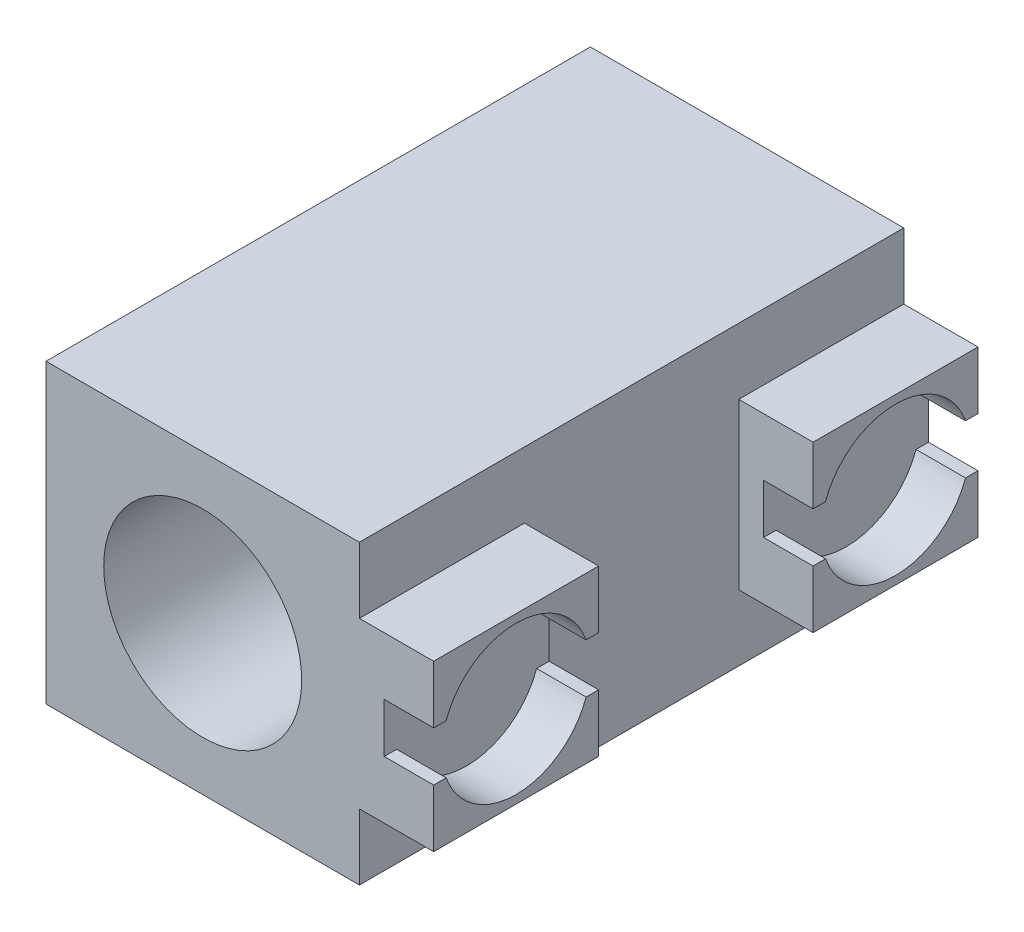
ISO-10303-21;
HEADER;
FILE_DESCRIPTION(('STEP AP214'),'2;1');
FILE_NAME('part.step','',(''),(''),'','','');
FILE_SCHEMA(('AUTOMOTIVE_DESIGN { 1 0 10303 214 1 1 1 1 }'));
ENDSEC;
DATA;
#1=APPLICATION_CONTEXT('core data for automotive mechanical design processes');
#2=APPLICATION_PROTOCOL_DEFINITION('international standard','automotive_design',2000,#1);
#3=PRODUCT_CONTEXT('',#1,'mechanical');
#4=PRODUCT('Part','Part','',(#3));
#5=PRODUCT_RELATED_PRODUCT_CATEGORY('part','',(#4));
#6=PRODUCT_DEFINITION_FORMATION('','',#4);
#7=PRODUCT_DEFINITION_CONTEXT('part definition',#1,'design');
#8=PRODUCT_DEFINITION('design','',#6,#7);
#9=PRODUCT_DEFINITION_SHAPE('','',#8);
#10=(LENGTH_UNIT() NAMED_UNIT(*) SI_UNIT(.MILLI.,.METRE.));
#11=(NAMED_UNIT(*) PLANE_ANGLE_UNIT() SI_UNIT($,.RADIAN.));
#12=(NAMED_UNIT(*) SI_UNIT($,.STERADIAN.) SOLID_ANGLE_UNIT());
#13=UNCERTAINTY_MEASURE_WITH_UNIT(LENGTH_MEASURE(1.E-05),#10,'distance_accuracy_value','');
#14=(GEOMETRIC_REPRESENTATION_CONTEXT(3) GLOBAL_UNCERTAINTY_ASSIGNED_CONTEXT((#13)) GLOBAL_UNIT_ASSIGNED_CONTEXT((#10,
#11,#12)) REPRESENTATION_CONTEXT('',''));
#15=CARTESIAN_POINT('',(0.,0.,0.));
#16=DIRECTION('',(0.,0.,1.));
#17=DIRECTION('',(1.,0.,0.));
#18=AXIS2_PLACEMENT_3D('',#15,#16,#17);
#19=CARTESIAN_POINT('',(47.,0.,0.));
#20=DIRECTION('',(1.,0.,0.));
#21=DIRECTION('',(0.,0.,-1.));
#22=AXIS2_PLACEMENT_3D('',#19,#20,#21);
#23=PLANE('',#22);
#24=DIRECTION('',(0.,0.,1.));
#25=VECTOR('',#24,1.);
#26=CARTESIAN_POINT('',(47.,-3.,-19.));
#27=LINE('',#26,#25);
#28=CARTESIAN_POINT('',(47.,-3.,-14.5147186257614));
#29=VERTEX_POINT('',#28);
#30=CARTESIAN_POINT('',(47.,-3.,-13.));
#31=VERTEX_POINT('',#30);
#32=EDGE_CURVE('E445',#29,#31,#27,.T.);
#33=ORIENTED_EDGE('',*,*,#32,.T.);
#34=DIRECTION('',(0.,-1.,0.));
#35=VECTOR('',#34,1.);
#36=CARTESIAN_POINT('',(47.,10.,-13.));
#37=LINE('',#36,#35);
#38=CARTESIAN_POINT('',(47.,-9.99999999999999,-13.));
#39=VERTEX_POINT('',#38);
#40=EDGE_CURVE('E258',#31,#39,#37,.T.);
#41=ORIENTED_EDGE('',*,*,#40,.T.);
#42=DIRECTION('',(0.,0.,-1.));
#43=VECTOR('',#42,1.);
#44=CARTESIAN_POINT('',(47.,-9.99999999999999,-13.));
#45=LINE('',#44,#43);
#46=CARTESIAN_POINT('',(47.,-9.99999999999999,-33.));
#47=VERTEX_POINT('',#46);
#48=EDGE_CURVE('E275',#39,#47,#45,.T.);
#49=ORIENTED_EDGE('',*,*,#48,.T.);
#50=DIRECTION('',(0.,1.,0.));
#51=VECTOR('',#50,1.);
#52=CARTESIAN_POINT('',(47.,-9.99999999999999,-33.));
#53=LINE('',#52,#51);
#54=CARTESIAN_POINT('',(47.,-3.,-33.));
#55=VERTEX_POINT('',#54);
#56=EDGE_CURVE('E421',#47,#55,#53,.T.);
#57=ORIENTED_EDGE('',*,*,#56,.T.);
#58=DIRECTION('',(0.,0.,-1.));
#59=VECTOR('',#58,1.);
#60=CARTESIAN_POINT('',(47.,-3.,-27.));
#61=LINE('',#60,#59);
#62=CARTESIAN_POINT('',(47.,-3.,-31.4852813742386));
#63=VERTEX_POINT('',#62);
#64=EDGE_CURVE('E463',#63,#55,#61,.T.);
#65=ORIENTED_EDGE('',*,*,#64,.F.);
#66=CARTESIAN_POINT('',(47.,0.,-23.));
#67=DIRECTION('',(1.,0.,0.));
#68=DIRECTION('',(0.,0.,-1.));
#69=AXIS2_PLACEMENT_3D('',#66,#67,#68);
#70=CIRCLE('',#69,9.);
#71=EDGE_CURVE('E475',#29,#63,#70,.T.);
#72=ORIENTED_EDGE('',*,*,#71,.F.);
#73=EDGE_LOOP('',(#33,#41,#49,#57,#65,#72));
#74=FACE_BOUND('',#73,.T.);
#75=ADVANCED_FACE('F39',(#74),#23,.T.);
#76=CARTESIAN_POINT('',(41.,0.,-23.));
#77=DIRECTION('',(1.,0.,0.));
#78=DIRECTION('',(0.,0.,-1.));
#79=AXIS2_PLACEMENT_3D('',#76,#77,#78);
#80=CYLINDRICAL_SURFACE('',#79,9.);
#81=CARTESIAN_POINT('',(41.,0.,-23.));
#82=DIRECTION('',(1.,0.,0.));
#83=DIRECTION('',(0.,0.,-1.));
#84=AXIS2_PLACEMENT_3D('',#81,#82,#83);
#85=CIRCLE('',#84,9.);
#86=CARTESIAN_POINT('',(41.,-3.,-14.5147186257614));
#87=VERTEX_POINT('',#86);
#88=CARTESIAN_POINT('',(41.,-3.,-31.4852813742386));
#89=VERTEX_POINT('',#88);
#90=EDGE_CURVE('E476',#87,#89,#85,.T.);
#91=ORIENTED_EDGE('',*,*,#90,.F.);
#92=DIRECTION('',(1.,0.,0.));
#93=VECTOR('',#92,1.);
#94=CARTESIAN_POINT('',(41.,-3.,-14.5147186257614));
#95=LINE('',#94,#93);
#96=EDGE_CURVE('E454',#87,#29,#95,.T.);
#97=ORIENTED_EDGE('',*,*,#96,.T.);
#98=ORIENTED_EDGE('',*,*,#71,.T.);
#99=DIRECTION('',(1.,0.,0.));
#100=VECTOR('',#99,1.);
#101=CARTESIAN_POINT('',(41.,-3.,-31.4852813742386));
#102=LINE('',#101,#100);
#103=EDGE_CURVE('E473',#63,#89,#102,.F.);
#104=ORIENTED_EDGE('',*,*,#103,.T.);
#105=EDGE_LOOP('',(#91,#97,#98,#104));
#106=FACE_BOUND('',#105,.T.);
#107=ADVANCED_FACE('F543',(#106),#80,.F.);
#108=CARTESIAN_POINT('',(47.,0.,0.));
#109=DIRECTION('',(-1.,0.,0.));
#110=DIRECTION('',(0.,0.,1.));
#111=AXIS2_PLACEMENT_3D('',#108,#109,#110);
#112=PLANE('',#111);
#113=DIRECTION('',(0.,1.,0.));
#114=VECTOR('',#113,1.);
#115=CARTESIAN_POINT('',(47.,10.,13.));
#116=LINE('',#115,#114);
#117=CARTESIAN_POINT('',(47.,-9.99999999999999,13.));
#118=VERTEX_POINT('',#117);
#119=CARTESIAN_POINT('',(47.,-3.,13.));
#120=VERTEX_POINT('',#119);
#121=EDGE_CURVE('E289',#118,#120,#116,.T.);
#122=ORIENTED_EDGE('',*,*,#121,.T.);
#123=DIRECTION('',(0.,0.,-1.));
#124=VECTOR('',#123,1.);
#125=CARTESIAN_POINT('',(47.,-3.,19.));
#126=LINE('',#125,#124);
#127=CARTESIAN_POINT('',(47.,-3.,14.5147186257614));
#128=VERTEX_POINT('',#127);
#129=EDGE_CURVE('E491',#128,#120,#126,.T.);
#130=ORIENTED_EDGE('',*,*,#129,.F.);
#131=CARTESIAN_POINT('',(47.,0.,23.));
#132=DIRECTION('',(1.,0.,0.));
#133=DIRECTION('',(0.,0.,-1.));
#134=AXIS2_PLACEMENT_3D('',#131,#132,#133);
#135=CIRCLE('',#134,9.);
#136=CARTESIAN_POINT('',(47.,-3.,31.4852813742386));
#137=VERTEX_POINT('',#136);
#138=EDGE_CURVE('E416',#137,#128,#135,.T.);
#139=ORIENTED_EDGE('',*,*,#138,.F.);
#140=DIRECTION('',(0.,0.,-1.));
#141=VECTOR('',#140,1.);
#142=CARTESIAN_POINT('',(47.,-3.,226.327850741589));
#143=LINE('',#142,#141);
#144=CARTESIAN_POINT('',(47.,-3.,33.));
#145=VERTEX_POINT('',#144);
#146=EDGE_CURVE('E376',#145,#137,#143,.T.);
#147=ORIENTED_EDGE('',*,*,#146,.F.);
#148=DIRECTION('',(0.,-1.,0.));
#149=VECTOR('',#148,1.);
#150=CARTESIAN_POINT('',(47.,-10.,33.));
#151=LINE('',#150,#149);
#152=CARTESIAN_POINT('',(47.,-10.,33.));
#153=VERTEX_POINT('',#152);
#154=EDGE_CURVE('E281',#145,#153,#151,.T.);
#155=ORIENTED_EDGE('',*,*,#154,.T.);
#156=DIRECTION('',(0.,0.,-1.));
#157=VECTOR('',#156,1.);
#158=CARTESIAN_POINT('',(47.,-9.99999999999999,13.));
#159=LINE('',#158,#157);
#160=EDGE_CURVE('E285',#153,#118,#159,.T.);
#161=ORIENTED_EDGE('',*,*,#160,.T.);
#162=EDGE_LOOP('',(#122,#130,#139,#147,#155,#161));
#163=FACE_BOUND('',#162,.T.);
#164=ADVANCED_FACE('F375',(#163),#112,.F.);
#165=CARTESIAN_POINT('',(41.,0.,23.));
#166=DIRECTION('',(1.,0.,0.));
#167=DIRECTION('',(0.,0.,-1.));
#168=AXIS2_PLACEMENT_3D('',#165,#166,#167);
#169=CYLINDRICAL_SURFACE('',#168,9.);
#170=ORIENTED_EDGE('',*,*,#138,.T.);
#171=DIRECTION('',(1.,0.,0.));
#172=VECTOR('',#171,1.);
#173=CARTESIAN_POINT('',(41.,-3.,14.5147186257614));
#174=LINE('',#173,#172);
#175=CARTESIAN_POINT('',(41.,-3.,14.5147186257614));
#176=VERTEX_POINT('',#175);
#177=EDGE_CURVE('E390',#128,#176,#174,.F.);
#178=ORIENTED_EDGE('',*,*,#177,.T.);
#179=CARTESIAN_POINT('',(41.,0.,23.));
#180=DIRECTION('',(1.,0.,0.));
#181=DIRECTION('',(0.,0.,-1.));
#182=AXIS2_PLACEMENT_3D('',#179,#180,#181);
#183=CIRCLE('',#182,9.);
#184=CARTESIAN_POINT('',(41.,-3.,31.4852813742386));
#185=VERTEX_POINT('',#184);
#186=EDGE_CURVE('E268',#185,#176,#183,.T.);
#187=ORIENTED_EDGE('',*,*,#186,.F.);
#188=DIRECTION('',(1.,0.,0.));
#189=VECTOR('',#188,1.);
#190=CARTESIAN_POINT('',(41.,-3.,31.4852813742386));
#191=LINE('',#190,#189);
#192=EDGE_CURVE('E414',#137,#185,#191,.F.);
#193=ORIENTED_EDGE('',*,*,#192,.F.);
#194=EDGE_LOOP('',(#170,#178,#187,#193));
#195=FACE_BOUND('',#194,.T.);
#196=ADVANCED_FACE('F530',(#195),#169,.F.);
#197=CARTESIAN_POINT('',(47.,3.,14.5147186257614));
#198=VERTEX_POINT('',#197);
#199=CARTESIAN_POINT('',(47.,3.,31.4852813742386));
#200=VERTEX_POINT('',#199);
#201=EDGE_CURVE('E415',#198,#200,#135,.T.);
#202=ORIENTED_EDGE('',*,*,#201,.F.);
#203=DIRECTION('',(0.,0.,-1.));
#204=VECTOR('',#203,1.);
#205=CARTESIAN_POINT('',(47.,3.,19.));
#206=LINE('',#205,#204);
#207=CARTESIAN_POINT('',(47.,3.,13.));
#208=VERTEX_POINT('',#207);
#209=EDGE_CURVE('E492',#198,#208,#206,.T.);
#210=ORIENTED_EDGE('',*,*,#209,.T.);
#211=CARTESIAN_POINT('',(47.,10.,13.));
#212=VERTEX_POINT('',#211);
#213=EDGE_CURVE('E288',#208,#212,#116,.T.);
#214=ORIENTED_EDGE('',*,*,#213,.T.);
#215=DIRECTION('',(0.,0.,1.));
#216=VECTOR('',#215,1.);
#217=CARTESIAN_POINT('',(47.,10.,33.));
#218=LINE('',#217,#216);
#219=CARTESIAN_POINT('',(47.,10.,33.));
#220=VERTEX_POINT('',#219);
#221=EDGE_CURVE('E286',#212,#220,#218,.T.);
#222=ORIENTED_EDGE('',*,*,#221,.T.);
#223=CARTESIAN_POINT('',(47.,3.,33.));
#224=VERTEX_POINT('',#223);
#225=EDGE_CURVE('E278',#220,#224,#151,.T.);
#226=ORIENTED_EDGE('',*,*,#225,.T.);
#227=DIRECTION('',(0.,0.,-1.));
#228=VECTOR('',#227,1.);
#229=CARTESIAN_POINT('',(47.,3.,226.327850741589));
#230=LINE('',#229,#228);
#231=EDGE_CURVE('E400',#224,#200,#230,.T.);
#232=ORIENTED_EDGE('',*,*,#231,.T.);
#233=EDGE_LOOP('',(#202,#210,#214,#222,#226,#232));
#234=FACE_BOUND('',#233,.T.);
#235=ADVANCED_FACE('F503',(#234),#112,.F.);
#236=CARTESIAN_POINT('',(41.,3.,14.5147186257614));
#237=VERTEX_POINT('',#236);
#238=CARTESIAN_POINT('',(41.,3.,31.4852813742386));
#239=VERTEX_POINT('',#238);
#240=EDGE_CURVE('E417',#237,#239,#183,.T.);
#241=ORIENTED_EDGE('',*,*,#240,.F.);
#242=DIRECTION('',(1.,0.,0.));
#243=VECTOR('',#242,1.);
#244=CARTESIAN_POINT('',(41.,3.,14.5147186257614));
#245=LINE('',#244,#243);
#246=EDGE_CURVE('E394',#237,#198,#245,.T.);
#247=ORIENTED_EDGE('',*,*,#246,.T.);
#248=ORIENTED_EDGE('',*,*,#201,.T.);
#249=DIRECTION('',(1.,0.,0.));
#250=VECTOR('',#249,1.);
#251=CARTESIAN_POINT('',(41.,3.,31.4852813742386));
#252=LINE('',#251,#250);
#253=EDGE_CURVE('E406',#239,#200,#252,.T.);
#254=ORIENTED_EDGE('',*,*,#253,.F.);
#255=EDGE_LOOP('',(#241,#247,#248,#254));
#256=FACE_BOUND('',#255,.T.);
#257=ADVANCED_FACE('F498',(#256),#169,.F.);
#258=CARTESIAN_POINT('',(38.,0.,0.));
#259=DIRECTION('',(1.,0.,0.));
#260=DIRECTION('',(0.,0.,-1.));
#261=AXIS2_PLACEMENT_3D('',#258,#259,#260);
#262=PLANE('',#261);
#263=DIRECTION('',(0.,1.,0.));
#264=VECTOR('',#263,1.);
#265=CARTESIAN_POINT('',(38.,18.,-33.));
#266=LINE('',#265,#264);
#267=CARTESIAN_POINT('',(38.,-18.,-33.));
#268=VERTEX_POINT('',#267);
#269=CARTESIAN_POINT('',(38.,-9.99999999999999,-33.));
#270=VERTEX_POINT('',#269);
#271=EDGE_CURVE('E311',#268,#270,#266,.T.);
#272=ORIENTED_EDGE('',*,*,#271,.T.);
#273=DIRECTION('',(0.,0.,-1.));
#274=VECTOR('',#273,1.);
#275=CARTESIAN_POINT('',(38.,-9.99999999999999,-13.));
#276=LINE('',#275,#274);
#277=CARTESIAN_POINT('',(38.,-9.99999999999999,-13.));
#278=VERTEX_POINT('',#277);
#279=EDGE_CURVE('E262',#278,#270,#276,.T.);
#280=ORIENTED_EDGE('',*,*,#279,.F.);
#281=DIRECTION('',(0.,-1.,0.));
#282=VECTOR('',#281,1.);
#283=CARTESIAN_POINT('',(38.,10.,-13.));
#284=LINE('',#283,#282);
#285=CARTESIAN_POINT('',(38.,10.,-13.));
#286=VERTEX_POINT('',#285);
#287=EDGE_CURVE('E271',#286,#278,#284,.T.);
#288=ORIENTED_EDGE('',*,*,#287,.F.);
#289=DIRECTION('',(0.,0.,1.));
#290=VECTOR('',#289,1.);
#291=CARTESIAN_POINT('',(38.,10.,-33.));
#292=LINE('',#291,#290);
#293=CARTESIAN_POINT('',(38.,10.,-33.));
#294=VERTEX_POINT('',#293);
#295=EDGE_CURVE('E270',#294,#286,#292,.T.);
#296=ORIENTED_EDGE('',*,*,#295,.F.);
#297=CARTESIAN_POINT('',(38.,18.,-33.));
#298=VERTEX_POINT('',#297);
#299=EDGE_CURVE('E320',#294,#298,#266,.T.);
#300=ORIENTED_EDGE('',*,*,#299,.T.);
#301=DIRECTION('',(0.,0.,1.));
#302=VECTOR('',#301,1.);
#303=CARTESIAN_POINT('',(38.,18.,33.));
#304=LINE('',#303,#302);
#305=CARTESIAN_POINT('',(38.,18.,33.));
#306=VERTEX_POINT('',#305);
#307=EDGE_CURVE('E316',#298,#306,#304,.T.);
#308=ORIENTED_EDGE('',*,*,#307,.T.);
#309=DIRECTION('',(0.,-1.,0.));
#310=VECTOR('',#309,1.);
#311=CARTESIAN_POINT('',(38.,18.,33.));
#312=LINE('',#311,#310);
#313=CARTESIAN_POINT('',(38.,10.,33.));
#314=VERTEX_POINT('',#313);
#315=EDGE_CURVE('E319',#306,#314,#312,.T.);
#316=ORIENTED_EDGE('',*,*,#315,.T.);
#317=DIRECTION('',(0.,0.,1.));
#318=VECTOR('',#317,1.);
#319=CARTESIAN_POINT('',(38.,10.,33.));
#320=LINE('',#319,#318);
#321=CARTESIAN_POINT('',(38.,10.,13.));
#322=VERTEX_POINT('',#321);
#323=EDGE_CURVE('E300',#322,#314,#320,.T.);
#324=ORIENTED_EDGE('',*,*,#323,.F.);
#325=DIRECTION('',(0.,1.,0.));
#326=VECTOR('',#325,1.);
#327=CARTESIAN_POINT('',(38.,10.,13.));
#328=LINE('',#327,#326);
#329=CARTESIAN_POINT('',(38.,-9.99999999999999,13.));
#330=VERTEX_POINT('',#329);
#331=EDGE_CURVE('E293',#330,#322,#328,.T.);
#332=ORIENTED_EDGE('',*,*,#331,.F.);
#333=DIRECTION('',(0.,0.,-1.));
#334=VECTOR('',#333,1.);
#335=CARTESIAN_POINT('',(38.,-9.99999999999999,13.));
#336=LINE('',#335,#334);
#337=CARTESIAN_POINT('',(38.,-10.,33.));
#338=VERTEX_POINT('',#337);
#339=EDGE_CURVE('E276',#338,#330,#336,.T.);
#340=ORIENTED_EDGE('',*,*,#339,.F.);
#341=CARTESIAN_POINT('',(38.,-18.,33.));
#342=VERTEX_POINT('',#341);
#343=EDGE_CURVE('E317',#338,#342,#312,.T.);
#344=ORIENTED_EDGE('',*,*,#343,.T.);
#345=DIRECTION('',(0.,0.,-1.));
#346=VECTOR('',#345,1.);
#347=CARTESIAN_POINT('',(38.,-18.,33.));
#348=LINE('',#347,#346);
#349=EDGE_CURVE('E325',#342,#268,#348,.T.);
#350=ORIENTED_EDGE('',*,*,#349,.T.);
#351=EDGE_LOOP('',(#272,#280,#288,#296,#300,#308,#316,#324,#332,#340,#344,#350));
#352=FACE_BOUND('',#351,.T.);
#353=ADVANCED_FACE('F362',(#352),#262,.T.);
#354=CARTESIAN_POINT('',(38.,18.,-33.));
#355=DIRECTION('',(0.,0.,1.));
#356=DIRECTION('',(1.,0.,0.));
#357=AXIS2_PLACEMENT_3D('',#354,#355,#356);
#358=PLANE('',#357);
#359=CARTESIAN_POINT('',(19.,0.,-33.));
#360=DIRECTION('',(0.,0.,1.));
#361=DIRECTION('',(1.,0.,0.));
#362=AXIS2_PLACEMENT_3D('',#359,#360,#361);
#363=CIRCLE('',#362,12.);
#364=CARTESIAN_POINT('',(31.,0.,-33.));
#365=VERTEX_POINT('',#364);
#366=EDGE_CURVE('E250',#365,#365,#363,.T.);
#367=ORIENTED_EDGE('',*,*,#366,.T.);
#368=EDGE_LOOP('',(#367));
#369=FACE_BOUND('',#368,.T.);
#370=DIRECTION('',(0.,1.,0.));
#371=VECTOR('',#370,1.);
#372=CARTESIAN_POINT('',(41.,0.,-33.));
#373=LINE('',#372,#371);
#374=CARTESIAN_POINT('',(41.,-3.,-33.));
#375=VERTEX_POINT('',#374);
#376=CARTESIAN_POINT('',(41.,3.,-33.));
#377=VERTEX_POINT('',#376);
#378=EDGE_CURVE('E451',#375,#377,#373,.T.);
#379=ORIENTED_EDGE('',*,*,#378,.F.);
#380=DIRECTION('',(-1.,0.,0.));
#381=VECTOR('',#380,1.);
#382=CARTESIAN_POINT('',(47.,-3.,-33.));
#383=LINE('',#382,#381);
#384=EDGE_CURVE('E459',#55,#375,#383,.T.);
#385=ORIENTED_EDGE('',*,*,#384,.F.);
#386=ORIENTED_EDGE('',*,*,#56,.F.);
#387=DIRECTION('',(-1.,0.,0.));
#388=VECTOR('',#387,1.);
#389=CARTESIAN_POINT('',(47.,-9.99999999999999,-33.));
#390=LINE('',#389,#388);
#391=EDGE_CURVE('E280',#47,#270,#390,.T.);
#392=ORIENTED_EDGE('',*,*,#391,.T.);
#393=ORIENTED_EDGE('',*,*,#271,.F.);
#394=DIRECTION('',(-1.,0.,0.));
#395=VECTOR('',#394,1.);
#396=CARTESIAN_POINT('',(38.,-18.,-33.));
#397=LINE('',#396,#395);
#398=CARTESIAN_POINT('',(0.,-18.,-33.));
#399=VERTEX_POINT('',#398);
#400=EDGE_CURVE('E322',#268,#399,#397,.T.);
#401=ORIENTED_EDGE('',*,*,#400,.T.);
#402=DIRECTION('',(0.,1.,0.));
#403=VECTOR('',#402,1.);
#404=CARTESIAN_POINT('',(0.,18.,-33.));
#405=LINE('',#404,#403);
#406=CARTESIAN_POINT('',(0.,18.,-33.));
#407=VERTEX_POINT('',#406);
#408=EDGE_CURVE('E315',#399,#407,#405,.T.);
#409=ORIENTED_EDGE('',*,*,#408,.T.);
#410=DIRECTION('',(-1.,0.,0.));
#411=VECTOR('',#410,1.);
#412=CARTESIAN_POINT('',(38.,18.,-33.));
#413=LINE('',#412,#411);
#414=EDGE_CURVE('E11',#298,#407,#413,.T.);
#415=ORIENTED_EDGE('',*,*,#414,.F.);
#416=ORIENTED_EDGE('',*,*,#299,.F.);
#417=DIRECTION('',(-1.,0.,0.));
#418=VECTOR('',#417,1.);
#419=CARTESIAN_POINT('',(47.,10.,-33.));
#420=LINE('',#419,#418);
#421=CARTESIAN_POINT('',(47.,10.,-33.));
#422=VERTEX_POINT('',#421);
#423=EDGE_CURVE('E274',#422,#294,#420,.T.);
#424=ORIENTED_EDGE('',*,*,#423,.F.);
#425=CARTESIAN_POINT('',(47.,3.,-33.));
#426=VERTEX_POINT('',#425);
#427=EDGE_CURVE('E425',#426,#422,#53,.T.);
#428=ORIENTED_EDGE('',*,*,#427,.F.);
#429=DIRECTION('',(1.,0.,0.));
#430=VECTOR('',#429,1.);
#431=CARTESIAN_POINT('',(41.,3.,-33.));
#432=LINE('',#431,#430);
#433=EDGE_CURVE('E460',#377,#426,#432,.T.);
#434=ORIENTED_EDGE('',*,*,#433,.F.);
#435=EDGE_LOOP('',(#379,#385,#386,#392,#393,#401,#409,#415,#416,#424,#428,#434));
#436=FACE_BOUND('',#435,.T.);
#437=ADVANCED_FACE('F41',(#369,#436),#358,.F.);
#438=CARTESIAN_POINT('',(38.,18.,33.));
#439=DIRECTION('',(0.,-1.,0.));
#440=DIRECTION('',(0.,0.,-1.));
#441=AXIS2_PLACEMENT_3D('',#438,#439,#440);
#442=PLANE('',#441);
#443=DIRECTION('',(0.,0.,1.));
#444=VECTOR('',#443,1.);
#445=CARTESIAN_POINT('',(0.,18.,33.));
#446=LINE('',#445,#444);
#447=CARTESIAN_POINT('',(0.,18.,33.));
#448=VERTEX_POINT('',#447);
#449=EDGE_CURVE('E330',#407,#448,#446,.T.);
#450=ORIENTED_EDGE('',*,*,#449,.T.);
#451=DIRECTION('',(-1.,0.,0.));
#452=VECTOR('',#451,1.);
#453=CARTESIAN_POINT('',(38.,18.,33.));
#454=LINE('',#453,#452);
#455=EDGE_CURVE('E50',#306,#448,#454,.T.);
#456=ORIENTED_EDGE('',*,*,#455,.F.);
#457=ORIENTED_EDGE('',*,*,#307,.F.);
#458=ORIENTED_EDGE('',*,*,#414,.T.);
#459=EDGE_LOOP('',(#450,#456,#457,#458));
#460=FACE_BOUND('',#459,.T.);
#461=ADVANCED_FACE('F535',(#460),#442,.F.);
#462=CARTESIAN_POINT('',(38.,18.,33.));
#463=DIRECTION('',(0.,0.,-1.));
#464=DIRECTION('',(-1.,0.,0.));
#465=AXIS2_PLACEMENT_3D('',#462,#463,#464);
#466=PLANE('',#465);
#467=CARTESIAN_POINT('',(19.,0.,33.));
#468=DIRECTION('',(0.,0.,1.));
#469=DIRECTION('',(1.,0.,0.));
#470=AXIS2_PLACEMENT_3D('',#467,#468,#469);
#471=CIRCLE('',#470,12.);
#472=CARTESIAN_POINT('',(31.,0.,33.));
#473=VERTEX_POINT('',#472);
#474=EDGE_CURVE('E797',#473,#473,#471,.T.);
#475=ORIENTED_EDGE('',*,*,#474,.F.);
#476=EDGE_LOOP('',(#475));
#477=FACE_BOUND('',#476,.T.);
#478=ORIENTED_EDGE('',*,*,#154,.F.);
#479=DIRECTION('',(-1.,0.,0.));
#480=VECTOR('',#479,1.);
#481=CARTESIAN_POINT('',(41.,-3.,33.));
#482=LINE('',#481,#480);
#483=CARTESIAN_POINT('',(41.,-3.,33.));
#484=VERTEX_POINT('',#483);
#485=EDGE_CURVE('E378',#145,#484,#482,.T.);
#486=ORIENTED_EDGE('',*,*,#485,.T.);
#487=DIRECTION('',(0.,1.,0.));
#488=VECTOR('',#487,1.);
#489=CARTESIAN_POINT('',(41.,0.,33.));
#490=LINE('',#489,#488);
#491=CARTESIAN_POINT('',(41.,0.,33.));
#492=VERTEX_POINT('',#491);
#493=EDGE_CURVE('E387',#484,#492,#490,.T.);
#494=ORIENTED_EDGE('',*,*,#493,.T.);
#495=DIRECTION('',(0.,1.,0.));
#496=VECTOR('',#495,1.);
#497=CARTESIAN_POINT('',(41.,0.,33.));
#498=LINE('',#497,#496);
#499=CARTESIAN_POINT('',(41.,3.,33.));
#500=VERTEX_POINT('',#499);
#501=EDGE_CURVE('E386',#492,#500,#498,.T.);
#502=ORIENTED_EDGE('',*,*,#501,.T.);
#503=DIRECTION('',(1.,0.,0.));
#504=VECTOR('',#503,1.);
#505=CARTESIAN_POINT('',(41.,3.,33.));
#506=LINE('',#505,#504);
#507=EDGE_CURVE('E399',#500,#224,#506,.T.);
#508=ORIENTED_EDGE('',*,*,#507,.T.);
#509=ORIENTED_EDGE('',*,*,#225,.F.);
#510=DIRECTION('',(-1.,0.,0.));
#511=VECTOR('',#510,1.);
#512=CARTESIAN_POINT('',(47.,10.,33.));
#513=LINE('',#512,#511);
#514=EDGE_CURVE('E295',#220,#314,#513,.T.);
#515=ORIENTED_EDGE('',*,*,#514,.T.);
#516=ORIENTED_EDGE('',*,*,#315,.F.);
#517=ORIENTED_EDGE('',*,*,#455,.T.);
#518=DIRECTION('',(0.,-1.,0.));
#519=VECTOR('',#518,1.);
#520=CARTESIAN_POINT('',(0.,18.,33.));
#521=LINE('',#520,#519);
#522=CARTESIAN_POINT('',(0.,-18.,33.));
#523=VERTEX_POINT('',#522);
#524=EDGE_CURVE('E328',#448,#523,#521,.T.);
#525=ORIENTED_EDGE('',*,*,#524,.T.);
#526=DIRECTION('',(-1.,0.,0.));
#527=VECTOR('',#526,1.);
#528=CARTESIAN_POINT('',(38.,-18.,33.));
#529=LINE('',#528,#527);
#530=EDGE_CURVE('E333',#342,#523,#529,.T.);
#531=ORIENTED_EDGE('',*,*,#530,.F.);
#532=ORIENTED_EDGE('',*,*,#343,.F.);
#533=DIRECTION('',(-1.,0.,0.));
#534=VECTOR('',#533,1.);
#535=CARTESIAN_POINT('',(47.,-10.,33.));
#536=LINE('',#535,#534);
#537=EDGE_CURVE('E310',#153,#338,#536,.T.);
#538=ORIENTED_EDGE('',*,*,#537,.F.);
#539=EDGE_LOOP('',(#478,#486,#494,#502,#508,#509,#515,#516,#517,#525,#531,#532,#538));
#540=FACE_BOUND('',#539,.T.);
#541=ADVANCED_FACE('F342',(#477,#540),#466,.F.);
#542=CARTESIAN_POINT('',(38.,-18.,33.));
#543=DIRECTION('',(0.,1.,0.));
#544=DIRECTION('',(0.,0.,1.));
#545=AXIS2_PLACEMENT_3D('',#542,#543,#544);
#546=PLANE('',#545);
#547=DIRECTION('',(0.,0.,-1.));
#548=VECTOR('',#547,1.);
#549=CARTESIAN_POINT('',(0.,-18.,33.));
#550=LINE('',#549,#548);
#551=EDGE_CURVE('E332',#523,#399,#550,.T.);
#552=ORIENTED_EDGE('',*,*,#551,.T.);
#553=ORIENTED_EDGE('',*,*,#400,.F.);
#554=ORIENTED_EDGE('',*,*,#349,.F.);
#555=ORIENTED_EDGE('',*,*,#530,.T.);
#556=EDGE_LOOP('',(#552,#553,#554,#555));
#557=FACE_BOUND('',#556,.T.);
#558=ADVANCED_FACE('F355',(#557),#546,.F.);
#559=CARTESIAN_POINT('',(0.,0.,0.));
#560=DIRECTION('',(1.,0.,0.));
#561=DIRECTION('',(0.,0.,-1.));
#562=AXIS2_PLACEMENT_3D('',#559,#560,#561);
#563=PLANE('',#562);
#564=ORIENTED_EDGE('',*,*,#408,.F.);
#565=ORIENTED_EDGE('',*,*,#551,.F.);
#566=ORIENTED_EDGE('',*,*,#524,.F.);
#567=ORIENTED_EDGE('',*,*,#449,.F.);
#568=EDGE_LOOP('',(#564,#565,#566,#567));
#569=FACE_BOUND('',#568,.T.);
#570=ADVANCED_FACE('F348',(#569),#563,.F.);
#571=CARTESIAN_POINT('',(47.,-9.99999999999999,13.));
#572=DIRECTION('',(0.,1.,0.));
#573=DIRECTION('',(0.,0.,1.));
#574=AXIS2_PLACEMENT_3D('',#571,#572,#573);
#575=PLANE('',#574);
#576=ORIENTED_EDGE('',*,*,#339,.T.);
#577=DIRECTION('',(-1.,0.,0.));
#578=VECTOR('',#577,1.);
#579=CARTESIAN_POINT('',(47.,-9.99999999999999,13.));
#580=LINE('',#579,#578);
#581=EDGE_CURVE('E308',#118,#330,#580,.T.);
#582=ORIENTED_EDGE('',*,*,#581,.F.);
#583=ORIENTED_EDGE('',*,*,#160,.F.);
#584=ORIENTED_EDGE('',*,*,#537,.T.);
#585=EDGE_LOOP('',(#576,#582,#583,#584));
#586=FACE_BOUND('',#585,.T.);
#587=ADVANCED_FACE('F366',(#586),#575,.F.);
#588=CARTESIAN_POINT('',(47.,10.,13.));
#589=DIRECTION('',(0.,0.,1.));
#590=DIRECTION('',(1.,0.,0.));
#591=AXIS2_PLACEMENT_3D('',#588,#589,#590);
#592=PLANE('',#591);
#593=DIRECTION('',(0.,1.,0.));
#594=VECTOR('',#593,1.);
#595=CARTESIAN_POINT('',(41.,0.,13.));
#596=LINE('',#595,#594);
#597=CARTESIAN_POINT('',(41.,-3.,13.));
#598=VERTEX_POINT('',#597);
#599=CARTESIAN_POINT('',(41.,3.,13.));
#600=VERTEX_POINT('',#599);
#601=EDGE_CURVE('E480',#598,#600,#596,.T.);
#602=ORIENTED_EDGE('',*,*,#601,.F.);
#603=DIRECTION('',(-1.,0.,0.));
#604=VECTOR('',#603,1.);
#605=CARTESIAN_POINT('',(47.,-3.,13.));
#606=LINE('',#605,#604);
#607=EDGE_CURVE('E484',#120,#598,#606,.T.);
#608=ORIENTED_EDGE('',*,*,#607,.F.);
#609=ORIENTED_EDGE('',*,*,#121,.F.);
#610=ORIENTED_EDGE('',*,*,#581,.T.);
#611=ORIENTED_EDGE('',*,*,#331,.T.);
#612=DIRECTION('',(-1.,0.,0.));
#613=VECTOR('',#612,1.);
#614=CARTESIAN_POINT('',(47.,10.,13.));
#615=LINE('',#614,#613);
#616=EDGE_CURVE('E302',#212,#322,#615,.T.);
#617=ORIENTED_EDGE('',*,*,#616,.F.);
#618=ORIENTED_EDGE('',*,*,#213,.F.);
#619=DIRECTION('',(1.,0.,0.));
#620=VECTOR('',#619,1.);
#621=CARTESIAN_POINT('',(41.,3.,13.));
#622=LINE('',#621,#620);
#623=EDGE_CURVE('E483',#600,#208,#622,.T.);
#624=ORIENTED_EDGE('',*,*,#623,.F.);
#625=EDGE_LOOP('',(#602,#608,#609,#610,#611,#617,#618,#624));
#626=FACE_BOUND('',#625,.T.);
#627=ADVANCED_FACE('F523',(#626),#592,.F.);
#628=CARTESIAN_POINT('',(47.,10.,33.));
#629=DIRECTION('',(0.,-1.,0.));
#630=DIRECTION('',(0.,0.,-1.));
#631=AXIS2_PLACEMENT_3D('',#628,#629,#630);
#632=PLANE('',#631);
#633=ORIENTED_EDGE('',*,*,#323,.T.);
#634=ORIENTED_EDGE('',*,*,#514,.F.);
#635=ORIENTED_EDGE('',*,*,#221,.F.);
#636=ORIENTED_EDGE('',*,*,#616,.T.);
#637=EDGE_LOOP('',(#633,#634,#635,#636));
#638=FACE_BOUND('',#637,.T.);
#639=ADVANCED_FACE('F527',(#638),#632,.F.);
#640=CARTESIAN_POINT('',(47.,-9.99999999999999,-13.));
#641=DIRECTION('',(0.,1.,0.));
#642=DIRECTION('',(0.,0.,1.));
#643=AXIS2_PLACEMENT_3D('',#640,#641,#642);
#644=PLANE('',#643);
#645=ORIENTED_EDGE('',*,*,#279,.T.);
#646=ORIENTED_EDGE('',*,*,#391,.F.);
#647=ORIENTED_EDGE('',*,*,#48,.F.);
#648=DIRECTION('',(-1.,0.,0.));
#649=VECTOR('',#648,1.);
#650=CARTESIAN_POINT('',(47.,-9.99999999999999,-13.));
#651=LINE('',#650,#649);
#652=EDGE_CURVE('E254',#39,#278,#651,.T.);
#653=ORIENTED_EDGE('',*,*,#652,.T.);
#654=EDGE_LOOP('',(#645,#646,#647,#653));
#655=FACE_BOUND('',#654,.T.);
#656=ADVANCED_FACE('F438',(#655),#644,.F.);
#657=CARTESIAN_POINT('',(47.,10.,-33.));
#658=DIRECTION('',(0.,-1.,0.));
#659=DIRECTION('',(0.,0.,-1.));
#660=AXIS2_PLACEMENT_3D('',#657,#658,#659);
#661=PLANE('',#660);
#662=ORIENTED_EDGE('',*,*,#295,.T.);
#663=DIRECTION('',(-1.,0.,0.));
#664=VECTOR('',#663,1.);
#665=CARTESIAN_POINT('',(47.,10.,-13.));
#666=LINE('',#665,#664);
#667=CARTESIAN_POINT('',(47.,10.,-13.));
#668=VERTEX_POINT('',#667);
#669=EDGE_CURVE('E259',#668,#286,#666,.T.);
#670=ORIENTED_EDGE('',*,*,#669,.F.);
#671=DIRECTION('',(0.,0.,1.));
#672=VECTOR('',#671,1.);
#673=CARTESIAN_POINT('',(47.,10.,-33.));
#674=LINE('',#673,#672);
#675=EDGE_CURVE('E251',#422,#668,#674,.T.);
#676=ORIENTED_EDGE('',*,*,#675,.F.);
#677=ORIENTED_EDGE('',*,*,#423,.T.);
#678=EDGE_LOOP('',(#662,#670,#676,#677));
#679=FACE_BOUND('',#678,.T.);
#680=ADVANCED_FACE('F434',(#679),#661,.F.);
#681=CARTESIAN_POINT('',(47.,10.,-13.));
#682=DIRECTION('',(0.,0.,-1.));
#683=DIRECTION('',(0.,1.,0.));
#684=AXIS2_PLACEMENT_3D('',#681,#682,#683);
#685=PLANE('',#684);
#686=ORIENTED_EDGE('',*,*,#40,.F.);
#687=DIRECTION('',(1.,0.,0.));
#688=VECTOR('',#687,1.);
#689=CARTESIAN_POINT('',(41.,-3.,-13.));
#690=LINE('',#689,#688);
#691=CARTESIAN_POINT('',(41.,-3.,-13.));
#692=VERTEX_POINT('',#691);
#693=EDGE_CURVE('E239',#692,#31,#690,.T.);
#694=ORIENTED_EDGE('',*,*,#693,.F.);
#695=DIRECTION('',(0.,-1.,0.));
#696=VECTOR('',#695,1.);
#697=CARTESIAN_POINT('',(41.,3.,-13.));
#698=LINE('',#697,#696);
#699=CARTESIAN_POINT('',(41.,3.,-13.));
#700=VERTEX_POINT('',#699);
#701=EDGE_CURVE('E247',#700,#692,#698,.T.);
#702=ORIENTED_EDGE('',*,*,#701,.F.);
#703=DIRECTION('',(-1.,0.,0.));
#704=VECTOR('',#703,1.);
#705=CARTESIAN_POINT('',(47.,3.,-13.));
#706=LINE('',#705,#704);
#707=CARTESIAN_POINT('',(47.,3.,-13.));
#708=VERTEX_POINT('',#707);
#709=EDGE_CURVE('E234',#708,#700,#706,.T.);
#710=ORIENTED_EDGE('',*,*,#709,.F.);
#711=EDGE_CURVE('E243',#668,#708,#37,.T.);
#712=ORIENTED_EDGE('',*,*,#711,.F.);
#713=ORIENTED_EDGE('',*,*,#669,.T.);
#714=ORIENTED_EDGE('',*,*,#287,.T.);
#715=ORIENTED_EDGE('',*,*,#652,.F.);
#716=EDGE_LOOP('',(#686,#694,#702,#710,#712,#713,#714,#715));
#717=FACE_BOUND('',#716,.T.);
#718=ADVANCED_FACE('F241',(#717),#685,.F.);
#719=DIRECTION('',(0.,0.,1.));
#720=VECTOR('',#719,1.);
#721=CARTESIAN_POINT('',(47.,3.,-19.));
#722=LINE('',#721,#720);
#723=CARTESIAN_POINT('',(47.,3.,-14.5147186257614));
#724=VERTEX_POINT('',#723);
#725=EDGE_CURVE('E226',#724,#708,#722,.T.);
#726=ORIENTED_EDGE('',*,*,#725,.F.);
#727=CARTESIAN_POINT('',(47.,3.,-31.4852813742386));
#728=VERTEX_POINT('',#727);
#729=EDGE_CURVE('E479',#728,#724,#70,.T.);
#730=ORIENTED_EDGE('',*,*,#729,.F.);
#731=DIRECTION('',(0.,0.,-1.));
#732=VECTOR('',#731,1.);
#733=CARTESIAN_POINT('',(47.,3.,-27.));
#734=LINE('',#733,#732);
#735=EDGE_CURVE('E429',#728,#426,#734,.T.);
#736=ORIENTED_EDGE('',*,*,#735,.T.);
#737=ORIENTED_EDGE('',*,*,#427,.T.);
#738=ORIENTED_EDGE('',*,*,#675,.T.);
#739=ORIENTED_EDGE('',*,*,#711,.T.);
#740=EDGE_LOOP('',(#726,#730,#736,#737,#738,#739));
#741=FACE_BOUND('',#740,.T.);
#742=ADVANCED_FACE('F253',(#741),#23,.T.);
#743=CARTESIAN_POINT('',(41.,0.,23.));
#744=DIRECTION('',(1.,0.,0.));
#745=DIRECTION('',(0.,0.,-1.));
#746=AXIS2_PLACEMENT_3D('',#743,#744,#745);
#747=PLANE('',#746);
#748=ORIENTED_EDGE('',*,*,#493,.F.);
#749=DIRECTION('',(0.,0.,-1.));
#750=VECTOR('',#749,1.);
#751=CARTESIAN_POINT('',(41.,-3.,226.327850741589));
#752=LINE('',#751,#750);
#753=EDGE_CURVE('E384',#484,#185,#752,.T.);
#754=ORIENTED_EDGE('',*,*,#753,.T.);
#755=ORIENTED_EDGE('',*,*,#186,.T.);
#756=DIRECTION('',(0.,0.,-1.));
#757=VECTOR('',#756,1.);
#758=CARTESIAN_POINT('',(41.,-3.,19.));
#759=LINE('',#758,#757);
#760=EDGE_CURVE('E488',#176,#598,#759,.T.);
#761=ORIENTED_EDGE('',*,*,#760,.T.);
#762=ORIENTED_EDGE('',*,*,#601,.T.);
#763=DIRECTION('',(0.,0.,-1.));
#764=VECTOR('',#763,1.);
#765=CARTESIAN_POINT('',(41.,3.,19.));
#766=LINE('',#765,#764);
#767=EDGE_CURVE('E490',#237,#600,#766,.T.);
#768=ORIENTED_EDGE('',*,*,#767,.F.);
#769=ORIENTED_EDGE('',*,*,#240,.T.);
#770=DIRECTION('',(0.,0.,-1.));
#771=VECTOR('',#770,1.);
#772=CARTESIAN_POINT('',(41.,3.,226.327850741589));
#773=LINE('',#772,#771);
#774=EDGE_CURVE('E405',#500,#239,#773,.T.);
#775=ORIENTED_EDGE('',*,*,#774,.F.);
#776=ORIENTED_EDGE('',*,*,#501,.F.);
#777=EDGE_LOOP('',(#748,#754,#755,#761,#762,#768,#769,#775,#776));
#778=FACE_BOUND('',#777,.T.);
#779=ADVANCED_FACE('F513',(#778),#747,.T.);
#780=CARTESIAN_POINT('',(41.,-3.,226.327850741589));
#781=DIRECTION('',(0.,1.,0.));
#782=DIRECTION('',(0.,0.,1.));
#783=AXIS2_PLACEMENT_3D('',#780,#781,#782);
#784=PLANE('',#783);
#785=ORIENTED_EDGE('',*,*,#146,.T.);
#786=ORIENTED_EDGE('',*,*,#192,.T.);
#787=ORIENTED_EDGE('',*,*,#753,.F.);
#788=ORIENTED_EDGE('',*,*,#485,.F.);
#789=EDGE_LOOP('',(#785,#786,#787,#788));
#790=FACE_BOUND('',#789,.T.);
#791=ADVANCED_FACE('F385',(#790),#784,.T.);
#792=CARTESIAN_POINT('',(41.,3.,226.327850741589));
#793=DIRECTION('',(0.,-1.,0.));
#794=DIRECTION('',(0.,0.,-1.));
#795=AXIS2_PLACEMENT_3D('',#792,#793,#794);
#796=PLANE('',#795);
#797=ORIENTED_EDGE('',*,*,#774,.T.);
#798=ORIENTED_EDGE('',*,*,#253,.T.);
#799=ORIENTED_EDGE('',*,*,#231,.F.);
#800=ORIENTED_EDGE('',*,*,#507,.F.);
#801=EDGE_LOOP('',(#797,#798,#799,#800));
#802=FACE_BOUND('',#801,.T.);
#803=ADVANCED_FACE('F512',(#802),#796,.T.);
#804=CARTESIAN_POINT('',(47.,-3.,19.));
#805=DIRECTION('',(0.,-1.,0.));
#806=DIRECTION('',(0.,0.,-1.));
#807=AXIS2_PLACEMENT_3D('',#804,#805,#806);
#808=PLANE('',#807);
#809=ORIENTED_EDGE('',*,*,#129,.T.);
#810=ORIENTED_EDGE('',*,*,#607,.T.);
#811=ORIENTED_EDGE('',*,*,#760,.F.);
#812=ORIENTED_EDGE('',*,*,#177,.F.);
#813=EDGE_LOOP('',(#809,#810,#811,#812));
#814=FACE_BOUND('',#813,.T.);
#815=ADVANCED_FACE('F533',(#814),#808,.F.);
#816=CARTESIAN_POINT('',(41.,3.,19.));
#817=DIRECTION('',(0.,1.,0.));
#818=DIRECTION('',(-1.,0.,0.));
#819=AXIS2_PLACEMENT_3D('',#816,#817,#818);
#820=PLANE('',#819);
#821=ORIENTED_EDGE('',*,*,#767,.T.);
#822=ORIENTED_EDGE('',*,*,#623,.T.);
#823=ORIENTED_EDGE('',*,*,#209,.F.);
#824=ORIENTED_EDGE('',*,*,#246,.F.);
#825=EDGE_LOOP('',(#821,#822,#823,#824));
#826=FACE_BOUND('',#825,.T.);
#827=ADVANCED_FACE('F516',(#826),#820,.F.);
#828=ORIENTED_EDGE('',*,*,#729,.T.);
#829=DIRECTION('',(1.,0.,0.));
#830=VECTOR('',#829,1.);
#831=CARTESIAN_POINT('',(41.,3.,-14.5147186257614));
#832=LINE('',#831,#830);
#833=CARTESIAN_POINT('',(41.,3.,-14.5147186257614));
#834=VERTEX_POINT('',#833);
#835=EDGE_CURVE('E235',#724,#834,#832,.F.);
#836=ORIENTED_EDGE('',*,*,#835,.T.);
#837=CARTESIAN_POINT('',(41.,3.,-31.4852813742386));
#838=VERTEX_POINT('',#837);
#839=EDGE_CURVE('E474',#838,#834,#85,.T.);
#840=ORIENTED_EDGE('',*,*,#839,.F.);
#841=DIRECTION('',(1.,0.,0.));
#842=VECTOR('',#841,1.);
#843=CARTESIAN_POINT('',(41.,3.,-31.4852813742386));
#844=LINE('',#843,#842);
#845=EDGE_CURVE('E461',#838,#728,#844,.T.);
#846=ORIENTED_EDGE('',*,*,#845,.T.);
#847=EDGE_LOOP('',(#828,#836,#840,#846));
#848=FACE_BOUND('',#847,.T.);
#849=ADVANCED_FACE('F552',(#848),#80,.F.);
#850=CARTESIAN_POINT('',(41.,0.,-23.));
#851=DIRECTION('',(1.,0.,0.));
#852=DIRECTION('',(0.,0.,-1.));
#853=AXIS2_PLACEMENT_3D('',#850,#851,#852);
#854=PLANE('',#853);
#855=ORIENTED_EDGE('',*,*,#839,.T.);
#856=DIRECTION('',(0.,0.,1.));
#857=VECTOR('',#856,1.);
#858=CARTESIAN_POINT('',(41.,3.,-19.));
#859=LINE('',#858,#857);
#860=EDGE_CURVE('E53',#834,#700,#859,.T.);
#861=ORIENTED_EDGE('',*,*,#860,.T.);
#862=ORIENTED_EDGE('',*,*,#701,.T.);
#863=DIRECTION('',(0.,0.,1.));
#864=VECTOR('',#863,1.);
#865=CARTESIAN_POINT('',(41.,-3.,-19.));
#866=LINE('',#865,#864);
#867=EDGE_CURVE('E450',#87,#692,#866,.T.);
#868=ORIENTED_EDGE('',*,*,#867,.F.);
#869=ORIENTED_EDGE('',*,*,#90,.T.);
#870=DIRECTION('',(0.,0.,-1.));
#871=VECTOR('',#870,1.);
#872=CARTESIAN_POINT('',(41.,-3.,-27.));
#873=LINE('',#872,#871);
#874=EDGE_CURVE('E464',#89,#375,#873,.T.);
#875=ORIENTED_EDGE('',*,*,#874,.T.);
#876=ORIENTED_EDGE('',*,*,#378,.T.);
#877=DIRECTION('',(0.,0.,-1.));
#878=VECTOR('',#877,1.);
#879=CARTESIAN_POINT('',(41.,3.,-27.));
#880=LINE('',#879,#878);
#881=EDGE_CURVE('E64',#838,#377,#880,.T.);
#882=ORIENTED_EDGE('',*,*,#881,.F.);
#883=EDGE_LOOP('',(#855,#861,#862,#868,#869,#875,#876,#882));
#884=FACE_BOUND('',#883,.T.);
#885=ADVANCED_FACE('F685',(#884),#854,.T.);
#886=CARTESIAN_POINT('',(47.,-3.,-27.));
#887=DIRECTION('',(0.,-1.,0.));
#888=DIRECTION('',(0.,0.,-1.));
#889=AXIS2_PLACEMENT_3D('',#886,#887,#888);
#890=PLANE('',#889);
#891=ORIENTED_EDGE('',*,*,#64,.T.);
#892=ORIENTED_EDGE('',*,*,#384,.T.);
#893=ORIENTED_EDGE('',*,*,#874,.F.);
#894=ORIENTED_EDGE('',*,*,#103,.F.);
#895=EDGE_LOOP('',(#891,#892,#893,#894));
#896=FACE_BOUND('',#895,.T.);
#897=ADVANCED_FACE('F679',(#896),#890,.F.);
#898=CARTESIAN_POINT('',(41.,3.,-27.));
#899=DIRECTION('',(0.,1.,0.));
#900=DIRECTION('',(0.,0.,1.));
#901=AXIS2_PLACEMENT_3D('',#898,#899,#900);
#902=PLANE('',#901);
#903=ORIENTED_EDGE('',*,*,#881,.T.);
#904=ORIENTED_EDGE('',*,*,#433,.T.);
#905=ORIENTED_EDGE('',*,*,#735,.F.);
#906=ORIENTED_EDGE('',*,*,#845,.F.);
#907=EDGE_LOOP('',(#903,#904,#905,#906));
#908=FACE_BOUND('',#907,.T.);
#909=ADVANCED_FACE('F684',(#908),#902,.F.);
#910=CARTESIAN_POINT('',(41.,-3.,-19.));
#911=DIRECTION('',(0.,-1.,0.));
#912=DIRECTION('',(1.,0.,0.));
#913=AXIS2_PLACEMENT_3D('',#910,#911,#912);
#914=PLANE('',#913);
#915=ORIENTED_EDGE('',*,*,#867,.T.);
#916=ORIENTED_EDGE('',*,*,#693,.T.);
#917=ORIENTED_EDGE('',*,*,#32,.F.);
#918=ORIENTED_EDGE('',*,*,#96,.F.);
#919=EDGE_LOOP('',(#915,#916,#917,#918));
#920=FACE_BOUND('',#919,.T.);
#921=ADVANCED_FACE('F692',(#920),#914,.F.);
#922=CARTESIAN_POINT('',(47.,3.,-19.));
#923=DIRECTION('',(0.,1.,0.));
#924=DIRECTION('',(-1.,0.,0.));
#925=AXIS2_PLACEMENT_3D('',#922,#923,#924);
#926=PLANE('',#925);
#927=ORIENTED_EDGE('',*,*,#725,.T.);
#928=ORIENTED_EDGE('',*,*,#709,.T.);
#929=ORIENTED_EDGE('',*,*,#860,.F.);
#930=ORIENTED_EDGE('',*,*,#835,.F.);
#931=EDGE_LOOP('',(#927,#928,#929,#930));
#932=FACE_BOUND('',#931,.T.);
#933=ADVANCED_FACE('F233',(#932),#926,.F.);
#934=CARTESIAN_POINT('',(19.,0.,-33.));
#935=DIRECTION('',(0.,0.,1.));
#936=DIRECTION('',(1.,0.,0.));
#937=AXIS2_PLACEMENT_3D('',#934,#935,#936);
#938=CYLINDRICAL_SURFACE('',#937,12.);
#939=ORIENTED_EDGE('',*,*,#366,.F.);
#940=EDGE_LOOP('',(#939));
#941=FACE_BOUND('',#940,.T.);
#942=ORIENTED_EDGE('',*,*,#474,.T.);
#943=EDGE_LOOP('',(#942));
#944=FACE_BOUND('',#943,.T.);
#945=ADVANCED_FACE('F732',(#941,#944),#938,.F.);
#946=CLOSED_SHELL('',(#75,#107,#164,#196,#235,#257,#353,#437,#461,#541,#558,#570,#587,#627,#639,
#656,#680,#718,#742,#779,#791,#803,#815,#827,#849,#885,#897,#909,#921,#933,#945));
#947=MANIFOLD_SOLID_BREP('B2',#946);
#948=ADVANCED_BREP_SHAPE_REPRESENTATION('',(#18,#947),#14);
#949=SHAPE_DEFINITION_REPRESENTATION(#9,#948);
ENDSEC;
END-ISO-10303-21;
